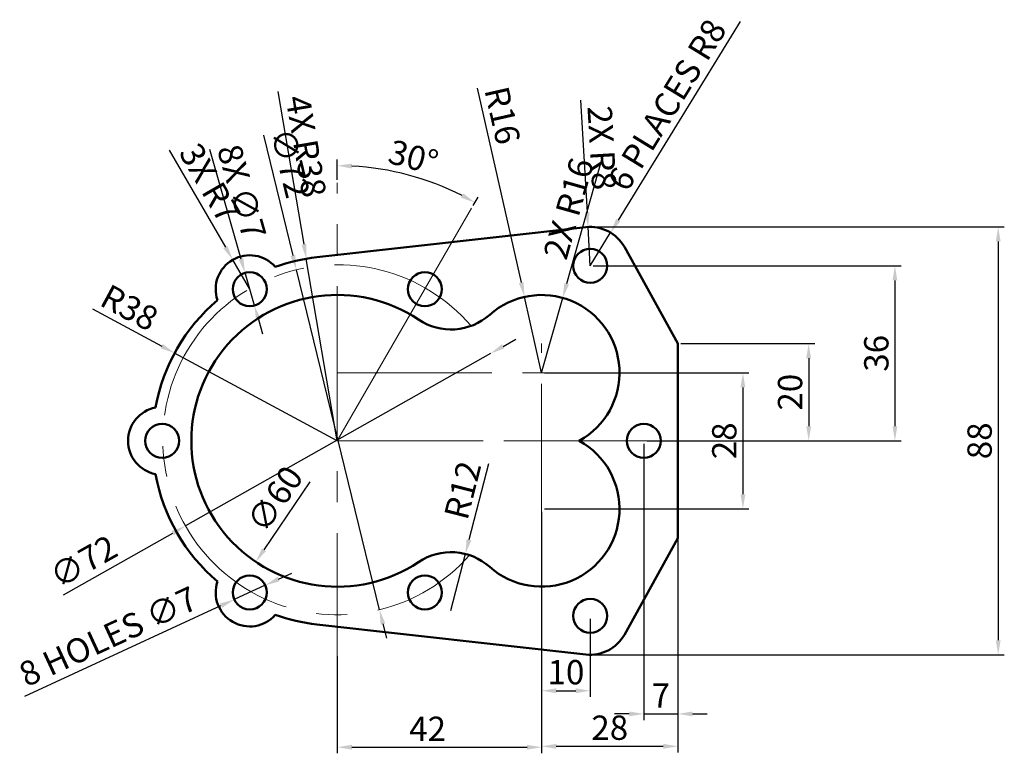
# Model space of a CAD drawing. Units: millimetres. Extents: x 620 to 823, y 325 to 476.
import ezdxf

# ---------------------------------------------------------------- set-up
doc = ezdxf.new("R2010")
doc.units = ezdxf.units.MM
doc.linetypes.add('CENTER', pattern=[50.8, 31.75, -6.35, 6.35, -6.35])
for name, color, linetype, lineweight in [('M-CNTR', 4, 'CENTER', 18), ('M-CONS', 8, 'Continuous', 18), ('M-DIMS', 2, 'Continuous', 25), ('M-OUTL', 7, 'Continuous', 50)]:
    doc.layers.add(name, color=color, linetype=linetype, lineweight=lineweight)
doc.styles.get("Standard").update_dxf_attribs({"font": 'arial.ttf'})
doc.dimstyles.new('ISO-25', dxfattribs={"dimtxt": 5, "dimasz": 3, "dimexe": 1.25, "dimexo": 0.625, "dimtad": 1, "dimdec": 0, "dimtxsty": 'Standard', "dimcen": 2.5, "dimadec": 0, "dimazin": 0, "dimtfac": 1, "dimtdec": 0, "dimtmove": 0, "dimatfit": 3, "dimfxl": 1, "dimarcsym": 0})

# ---------------------------------------------------------------- blocks, each defined once
blk = doc.blocks.new('*D1')
at = {"layer": 'Defpoints', "color": 0, "transparency": 16777216}
for p in [(737.47, 433.5), (737.47, 345.5), (821.32, 345.5)]:
    blk.add_point(p, dxfattribs=at)
at = {"layer": 'M-DIMS', "color": 0, "lineweight": -2, "transparency": 16777216}
for p, q in [((738.09, 433.5), (822.57, 433.5)), ((821.32, 430.5), (821.32, 348.5)), ((738.09, 345.5), (822.57, 345.5))]:
    blk.add_line(p, q, dxfattribs=at)
at = {"layer": 'M-DIMS', "color": 0, "transparency": 16777216}
for points in [[(820.82, 430.5), (821.82, 430.5), (821.32, 433.5)], [(820.82, 348.5), (821.82, 348.5), (821.32, 345.5)]]:
    blk.add_solid(points, dxfattribs=at)
at = {"layer": 'M-DIMS', "color": 0, "transparency": 16777216, "insert": (818.14, 389.5), "char_height": 5, "attachment_point": 5, "rotation": 90}
blk.add_mtext('88', dxfattribs=at)
blk = doc.blocks.new('*D2')
at = {"layer": 'Defpoints', "color": 0, "transparency": 16777216}
for p in [(737.47, 425.5), (748.54, 389.5), (800.09, 389.5)]:
    blk.add_point(p, dxfattribs=at)
at = {"layer": 'M-DIMS', "color": 0, "lineweight": -2, "transparency": 16777216}
for p, q in [((738.09, 425.5), (801.34, 425.5)), ((800.09, 422.5), (800.09, 392.5)), ((749.16, 389.5), (801.34, 389.5))]:
    blk.add_line(p, q, dxfattribs=at)
at = {"layer": 'M-DIMS', "color": 0, "transparency": 16777216}
for points in [[(799.59, 422.5), (800.59, 422.5), (800.09, 425.5)], [(799.59, 392.5), (800.59, 392.5), (800.09, 389.5)]]:
    blk.add_solid(points, dxfattribs=at)
at = {"layer": 'M-DIMS', "color": 0, "transparency": 16777216, "insert": (796.91, 407.5), "char_height": 5, "attachment_point": 5, "rotation": 90}
blk.add_mtext('36', dxfattribs=at)
blk = doc.blocks.new('*D3')
at = {"layer": 'Defpoints', "color": 0, "transparency": 16777216}
for p in [(727.47, 375.5), (685.47, 345.82), (727.47, 326.48)]:
    blk.add_point(p, dxfattribs=at)
at = {"layer": 'M-DIMS', "color": 0, "lineweight": -2, "transparency": 16777216}
for p, q in [((727.47, 374.87), (727.47, 325.23)), ((685.47, 345.2), (685.47, 325.23)), ((688.47, 326.48), (724.47, 326.48))]:
    blk.add_line(p, q, dxfattribs=at)
at = {"layer": 'M-DIMS', "color": 0, "transparency": 16777216}
for points in [[(688.47, 326.98), (688.47, 325.98), (685.47, 326.48)], [(724.47, 326.98), (724.47, 325.98), (727.47, 326.48)]]:
    blk.add_solid(points, dxfattribs=at)
at = {"layer": 'M-DIMS', "color": 0, "transparency": 16777216, "insert": (704.03, 329.62), "char_height": 5, "attachment_point": 5}
blk.add_mtext('42', dxfattribs=at)
blk = doc.blocks.new('*D4')
at = {"layer": 'Defpoints', "color": 0, "transparency": 16777216}
for p in [(755.47, 409.5), (763.47, 389.5), (782.36, 389.5)]:
    blk.add_point(p, dxfattribs=at)
at = {"layer": 'M-DIMS', "color": 0, "lineweight": -2, "transparency": 16777216}
for p, q in [((756.09, 409.5), (783.61, 409.5)), ((782.36, 406.5), (782.36, 392.5)), ((764.09, 389.5), (783.61, 389.5))]:
    blk.add_line(p, q, dxfattribs=at)
at = {"layer": 'M-DIMS', "color": 0, "transparency": 16777216}
for points in [[(781.86, 406.5), (782.86, 406.5), (782.36, 409.5)], [(781.86, 392.5), (782.86, 392.5), (782.36, 389.5)]]:
    blk.add_solid(points, dxfattribs=at)
at = {"layer": 'M-DIMS', "color": 0, "transparency": 16777216, "insert": (779.18, 399.5), "char_height": 5, "attachment_point": 5, "rotation": 90}
blk.add_mtext('20', dxfattribs=at)
blk = doc.blocks.new('*D5')
at = {"layer": 'Defpoints', "color": 0, "transparency": 16777216}
for p in [(727.47, 403.5), (727.47, 375.5), (768.84, 375.5)]:
    blk.add_point(p, dxfattribs=at)
at = {"layer": 'M-DIMS', "color": 0, "lineweight": -2, "transparency": 16777216}
for p, q in [((728.09, 403.5), (770.09, 403.5)), ((768.84, 400.5), (768.84, 378.5)), ((728.09, 375.5), (770.09, 375.5))]:
    blk.add_line(p, q, dxfattribs=at)
at = {"layer": 'M-DIMS', "color": 0, "transparency": 16777216}
for points in [[(768.34, 400.5), (769.34, 400.5), (768.84, 403.5)], [(768.34, 378.5), (769.34, 378.5), (768.84, 375.5)]]:
    blk.add_solid(points, dxfattribs=at)
at = {"layer": 'M-DIMS', "color": 0, "transparency": 16777216, "insert": (765.66, 389.5), "char_height": 5, "attachment_point": 5, "rotation": 90}
blk.add_mtext('28', dxfattribs=at)
blk = doc.blocks.new('*D6')
at = {"layer": 'Defpoints', "color": 0, "transparency": 16777216}
for p in [(748.47, 389.5), (755.47, 383.53), (755.47, 333.33)]:
    blk.add_point(p, dxfattribs=at)
at = {"layer": 'M-DIMS', "color": 0, "lineweight": -2, "transparency": 16777216}
for p, q in [((748.47, 388.87), (748.47, 332.08)), ((755.47, 382.9), (755.47, 332.08)), ((745.47, 333.33), (742.47, 333.33)), ((748.47, 333.33), (755.47, 333.33)), ((758.47, 333.33), (761.47, 333.33))]:
    blk.add_line(p, q, dxfattribs=at)
at = {"layer": 'M-DIMS', "color": 0, "transparency": 16777216}
for points in [[(745.47, 333.83), (745.47, 332.83), (748.47, 333.33)], [(758.47, 333.83), (758.47, 332.83), (755.47, 333.33)]]:
    blk.add_solid(points, dxfattribs=at)
at = {"layer": 'M-DIMS', "color": 0, "transparency": 16777216, "insert": (751.97, 336.46), "char_height": 5, "attachment_point": 5}
blk.add_mtext('7', dxfattribs=at)
blk = doc.blocks.new('*D7')
at = {"layer": 'Defpoints', "color": 0, "transparency": 16777216}
for p in [(737.47, 353.5), (727.47, 344.51), (737.47, 338.1)]:
    blk.add_point(p, dxfattribs=at)
at = {"layer": 'M-DIMS', "color": 0, "lineweight": -2, "transparency": 16777216}
for p, q in [((737.47, 352.87), (737.47, 336.85)), ((727.47, 343.88), (727.47, 336.85)), ((730.47, 338.1), (734.47, 338.1))]:
    blk.add_line(p, q, dxfattribs=at)
at = {"layer": 'M-DIMS', "color": 0, "transparency": 16777216}
for points in [[(730.47, 338.6), (730.47, 337.6), (727.47, 338.1)], [(734.47, 338.6), (734.47, 337.6), (737.47, 338.1)]]:
    blk.add_solid(points, dxfattribs=at)
at = {"layer": 'M-DIMS', "color": 0, "transparency": 16777216, "insert": (732.47, 341.27), "char_height": 5, "attachment_point": 5}
blk.add_mtext('10', dxfattribs=at)
blk = doc.blocks.new('*D8')
at = {"layer": 'Defpoints', "color": 0, "transparency": 16777216}
for p in [(741.65, 432.32), (737.47, 425.5)]:
    blk.add_point(p, dxfattribs=at)
at = {"layer": 'M-DIMS', "color": 0, "lineweight": -2, "transparency": 16777216}
for p, q in [((768.26, 475.75), (743.21, 434.88)), ((737.47, 425.5), (741.65, 432.32))]:
    blk.add_line(p, q, dxfattribs=at)
at = {"layer": 'M-DIMS', "color": 0, "transparency": 16777216}
blk.add_solid([(742.79, 435.14), (743.64, 434.62), (741.65, 432.32)], dxfattribs=at)
at = {"layer": 'M-DIMS', "color": 0, "transparency": 16777216, "insert": (753.78, 458.27), "char_height": 5, "attachment_point": 5, "rotation": 58.5023}
blk.add_mtext('6 PLACES R8', dxfattribs=at)
blk = doc.blocks.new('*D9')
at = {"layer": 'Defpoints', "color": 0, "transparency": 16777216}
for p in [(723.94, 419.1), (727.47, 403.5)]:
    blk.add_point(p, dxfattribs=at)
at = {"layer": 'M-DIMS', "color": 0, "lineweight": -2, "transparency": 16777216}
for p, q in [((714.23, 462.03), (723.28, 422.03)), ((727.47, 403.5), (723.94, 419.1))]:
    blk.add_line(p, q, dxfattribs=at)
at = {"layer": 'M-DIMS', "color": 0, "transparency": 16777216}
blk.add_solid([(723.76, 422.14), (722.79, 421.92), (723.94, 419.1)], dxfattribs=at)
at = {"layer": 'M-DIMS', "color": 0, "transparency": 16777216, "insert": (718.79, 456.3), "char_height": 5, "attachment_point": 5, "rotation": 282.7415}
blk.add_mtext('R16', dxfattribs=at)
blk = doc.blocks.new('*D10')
at = {"layer": 'Defpoints', "color": 0, "transparency": 16777216}
for p in [(711.79, 366.23), (708.83, 354.6)]:
    blk.add_point(p, dxfattribs=at)
at = {"layer": 'M-DIMS', "color": 0, "lineweight": -2, "transparency": 16777216}
for p, q in [((716.52, 384.78), (712.53, 369.13)), ((708.83, 354.6), (711.79, 366.23))]:
    blk.add_line(p, q, dxfattribs=at)
at = {"layer": 'M-DIMS', "color": 0, "transparency": 16777216}
blk.add_solid([(712.05, 369.26), (713.02, 369.01), (711.79, 366.23)], dxfattribs=at)
at = {"layer": 'M-DIMS', "color": 0, "transparency": 16777216, "insert": (711.86, 379.18), "char_height": 5, "attachment_point": 5, "rotation": 75.7174}
blk.add_mtext('R12', dxfattribs=at)
blk = doc.blocks.new('*D11')
at = {"layer": 'Defpoints', "color": 0, "transparency": 16777216}
for p in [(652.03, 407.54), (685.47, 389.5)]:
    blk.add_point(p, dxfattribs=at)
at = {"layer": 'M-DIMS', "color": 0, "lineweight": -2, "transparency": 16777216}
for p, q in [((635.12, 416.67), (649.39, 408.97)), ((685.47, 389.5), (652.03, 407.54))]:
    blk.add_line(p, q, dxfattribs=at)
at = {"layer": 'M-DIMS', "color": 0, "transparency": 16777216}
blk.add_solid([(649.62, 409.41), (649.15, 408.53), (652.03, 407.54)], dxfattribs=at)
at = {"layer": 'M-DIMS', "color": 0, "transparency": 16777216, "insert": (642.44, 416.33), "char_height": 5, "attachment_point": 5, "rotation": 331.6462}
blk.add_mtext('R38', dxfattribs=at)
blk = doc.blocks.new('*D12')
at = {"layer": 'Defpoints', "color": 0, "transparency": 16777216}
for p in [(716.93, 407.44), (654.26, 371.99)]:
    blk.add_point(p, dxfattribs=at)
at = {"layer": 'M-DIMS', "color": 0, "lineweight": -2, "transparency": 16777216}
for p, q in [((719.54, 408.92), (722.15, 410.4)), ((716.93, 407.44), (654.26, 371.99)), ((629.21, 357.82), (651.65, 370.52))]:
    blk.add_line(p, q, dxfattribs=at)
at = {"layer": 'M-DIMS', "color": 0, "transparency": 16777216}
for points in [[(719.29, 409.36), (719.79, 408.49), (716.93, 407.44)], [(651.4, 370.95), (651.9, 370.08), (654.26, 371.99)]]:
    blk.add_solid(points, dxfattribs=at)
at = {"layer": 'M-DIMS', "color": 0, "transparency": 16777216, "insert": (633.59, 364.11), "char_height": 5, "attachment_point": 5, "rotation": 29.4967}
blk.add_mtext('∅72', dxfattribs=at)
blk = doc.blocks.new('*D13')
at = {"layer": 'Defpoints', "color": 0, "transparency": 16777216}
for p in [(702.22, 414.39), (668.72, 364.61)]:
    blk.add_point(p, dxfattribs=at)
at = {"layer": 'M-DIMS', "color": 0, "lineweight": -2, "transparency": 16777216}
blk.add_line((679.79, 381.06), (670.39, 367.1), dxfattribs=at)
at = {"layer": 'M-DIMS', "color": 0, "transparency": 16777216}
blk.add_solid([(669.98, 367.38), (670.81, 366.82), (668.72, 364.61)], dxfattribs=at)
at = {"layer": 'M-DIMS', "color": 0, "transparency": 16777216, "insert": (673.18, 377.18), "char_height": 5, "attachment_point": 5, "rotation": 56.0608}
blk.add_mtext('∅60', dxfattribs=at)
blk = doc.blocks.new('*D14')
at = {"layer": 'Defpoints', "color": 0, "transparency": 16777216}
for p in [(670.65, 359.79), (664.29, 356.86)]:
    blk.add_point(p, dxfattribs=at)
at = {"layer": 'M-DIMS', "color": 0, "lineweight": -2, "transparency": 16777216}
for p, q in [((673.37, 361.04), (676.1, 362.3)), ((670.65, 359.79), (664.29, 356.86)), ((621.23, 337.01), (661.56, 355.6))]:
    blk.add_line(p, q, dxfattribs=at)
at = {"layer": 'M-DIMS', "color": 0, "transparency": 16777216}
for points in [[(673.16, 361.5), (673.58, 360.59), (670.65, 359.79)], [(661.35, 356.05), (661.77, 355.15), (664.29, 356.86)]]:
    blk.add_solid(points, dxfattribs=at)
at = {"layer": 'M-DIMS', "color": 0, "transparency": 16777216, "insert": (638.65, 348.69), "char_height": 5, "attachment_point": 5, "rotation": 24.7445}
blk.add_mtext('8 HOLES ∅7', dxfattribs=at)
blk = doc.blocks.new('*D15')
at = {"layer": 'Defpoints', "color": 0, "transparency": 16777216}
for p in [(685.47, 442.56), (704.82, 442.68), (713.08, 437.33), (685.47, 389.5), (685.47, 338.78)]:
    blk.add_point(p, dxfattribs=at)
at = {"layer": 'M-DIMS', "color": 0, "lineweight": -2, "transparency": 16777216}
for p, q in [((685.47, 443.18), (685.47, 447.34)), ((713.39, 437.87), (714.39, 439.59))]:
    blk.add_line(p, q, dxfattribs=at)
blk.add_arc((685.47, 389.5), 56.59, 63.0377, 86.9623, dxfattribs=at)
at = {"layer": 'M-DIMS', "color": 0, "transparency": 16777216}
for points in [[(688.45, 445.51), (688.48, 446.51), (685.47, 446.09)], [(711.36, 440.38), (710.89, 439.5), (713.76, 438.51)]]:
    blk.add_solid(points, dxfattribs=at)
at = {"layer": 'M-DIMS', "color": 0, "transparency": 16777216, "insert": (700.94, 447.23), "char_height": 5, "attachment_point": 5, "rotation": 345}
blk.add_mtext('30°', dxfattribs=at)
blk = doc.blocks.new('*D16')
at = {"layer": 'Defpoints', "color": 0, "transparency": 16777216}
for p in [(727.47, 343.1), (755.47, 343.1), (755.47, 326.67)]:
    blk.add_point(p, dxfattribs=at)
at = {"layer": 'M-DIMS', "color": 0, "lineweight": -2, "transparency": 16777216}
for p, q in [((727.47, 342.48), (727.47, 325.42)), ((755.47, 342.48), (755.47, 325.42)), ((730.47, 326.67), (752.47, 326.67))]:
    blk.add_line(p, q, dxfattribs=at)
at = {"layer": 'M-DIMS', "color": 0, "transparency": 16777216}
for points in [[(730.47, 327.17), (730.47, 326.17), (727.47, 326.67)], [(752.47, 327.17), (752.47, 326.17), (755.47, 326.67)]]:
    blk.add_solid(points, dxfattribs=at)
at = {"layer": 'M-DIMS', "color": 0, "transparency": 16777216, "insert": (741.47, 329.85), "char_height": 5, "attachment_point": 5}
blk.add_mtext('28', dxfattribs=at)
blk = doc.blocks.new('BOLT-HOLE-D7')
blk.add_circle((3.5, 3.5), 3.5)
blk = doc.blocks.new('*D18')
at = {"layer": 'Defpoints', "color": 0, "transparency": 16777216}
for p in [(666.5, 424.04), (668.43, 417.31)]:
    blk.add_point(p, dxfattribs=at)
at = {"layer": 'M-DIMS', "color": 0, "lineweight": -2, "transparency": 16777216}
for p, q in [((659.19, 449.46), (665.67, 426.92)), ((668.43, 417.31), (666.5, 424.04)), ((669.26, 414.43), (670.09, 411.54))]:
    blk.add_line(p, q, dxfattribs=at)
at = {"layer": 'M-DIMS', "color": 0, "transparency": 16777216}
for points in [[(666.15, 427.06), (665.19, 426.78), (666.5, 424.04)], [(669.74, 414.57), (668.78, 414.29), (668.43, 417.31)]]:
    blk.add_solid(points, dxfattribs=at)
at = {"layer": 'M-DIMS', "color": 0, "transparency": 16777216, "insert": (665.21, 440.55), "char_height": 5, "attachment_point": 5, "rotation": 286.0373}
blk.add_mtext('8X ∅7', dxfattribs=at)
blk = doc.blocks.new('*D19')
at = {"layer": 'Defpoints', "color": 0, "transparency": 16777216}
for p in [(663.97, 426.74), (667.47, 420.67)]:
    blk.add_point(p, dxfattribs=at)
at = {"layer": 'M-DIMS', "color": 0, "lineweight": -2, "transparency": 16777216}
for p, q in [((650.94, 449.3), (662.47, 429.33)), ((667.47, 420.67), (663.97, 426.74))]:
    blk.add_line(p, q, dxfattribs=at)
at = {"layer": 'M-DIMS', "color": 0, "transparency": 16777216}
blk.add_solid([(662.9, 429.58), (662.03, 429.08), (663.97, 426.74)], dxfattribs=at)
at = {"layer": 'M-DIMS', "color": 0, "transparency": 16777216, "insert": (658.71, 442.21), "char_height": 5, "attachment_point": 5, "rotation": 300.0017}
blk.add_mtext('3X R7', dxfattribs=at)
blk = doc.blocks.new('*D20')
at = {"layer": 'Defpoints', "color": 0, "transparency": 16777216}
for p in [(737, 433.48), (737.47, 425.5)]:
    blk.add_point(p, dxfattribs=at)
at = {"layer": 'M-DIMS', "color": 0, "lineweight": -2, "transparency": 16777216}
for p, q in [((735.47, 459.59), (736.82, 436.48)), ((737.47, 425.5), (737, 433.48))]:
    blk.add_line(p, q, dxfattribs=at)
at = {"layer": 'M-DIMS', "color": 0, "transparency": 16777216}
blk.add_solid([(737.32, 436.51), (736.33, 436.45), (737, 433.48)], dxfattribs=at)
at = {"layer": 'M-DIMS', "color": 0, "transparency": 16777216, "insert": (739.23, 449.72), "char_height": 5, "attachment_point": 5, "rotation": 273.351}
blk.add_mtext('2X R8', dxfattribs=at)
blk = doc.blocks.new('*D21')
at = {"layer": 'Defpoints', "color": 0, "transparency": 16777216}
for p in [(679.1, 426.96), (685.47, 389.5)]:
    blk.add_point(p, dxfattribs=at)
at = {"layer": 'M-DIMS', "color": 0, "lineweight": -2, "transparency": 16777216}
for p, q in [((673.25, 461.34), (678.6, 429.92)), ((685.47, 389.5), (679.1, 426.96))]:
    blk.add_line(p, q, dxfattribs=at)
at = {"layer": 'M-DIMS', "color": 0, "transparency": 16777216}
blk.add_solid([(679.09, 430), (678.1, 429.83), (679.1, 426.96)], dxfattribs=at)
at = {"layer": 'M-DIMS', "color": 0, "transparency": 16777216, "insert": (678.41, 449.97), "char_height": 5, "attachment_point": 5, "rotation": 279.6488}
blk.add_mtext('4X R38', dxfattribs=at)
blk = doc.blocks.new('*D22')
at = {"layer": 'Defpoints', "color": 0, "transparency": 16777216}
for p in [(677.05, 424.69), (694.14, 354.75)]:
    blk.add_point(p, dxfattribs=at)
at = {"layer": 'M-DIMS', "color": 0, "lineweight": -2, "transparency": 16777216}
for p, q in [((670.29, 452.38), (676.34, 427.6)), ((694.14, 354.75), (677.05, 424.69)), ((694.85, 351.83), (695.56, 348.92))]:
    blk.add_line(p, q, dxfattribs=at)
at = {"layer": 'M-DIMS', "color": 0, "transparency": 16777216}
for points in [[(676.82, 427.72), (675.85, 427.49), (677.05, 424.69)], [(695.34, 351.95), (694.37, 351.71), (694.14, 354.75)]]:
    blk.add_solid(points, dxfattribs=at)
at = {"layer": 'M-DIMS', "color": 0, "transparency": 16777216, "insert": (675.15, 446.46), "char_height": 5, "attachment_point": 5, "rotation": 283.7292}
blk.add_mtext('∅72', dxfattribs=at)
blk = doc.blocks.new('*D23')
at = {"layer": 'Defpoints', "color": 0, "transparency": 16777216}
for p in [(731.8, 418.9), (727.47, 403.5)]:
    blk.add_point(p, dxfattribs=at)
at = {"layer": 'M-DIMS', "color": 0, "lineweight": -2, "transparency": 16777216}
for p, q in [((739.93, 447.8), (732.61, 421.79)), ((727.47, 403.5), (731.8, 418.9))]:
    blk.add_line(p, q, dxfattribs=at)
at = {"layer": 'M-DIMS', "color": 0, "transparency": 16777216}
blk.add_solid([(732.13, 421.92), (733.09, 421.65), (731.8, 418.9)], dxfattribs=at)
at = {"layer": 'M-DIMS', "color": 0, "transparency": 16777216, "insert": (733.62, 437.1), "char_height": 5, "attachment_point": 5, "rotation": 74.289}
blk.add_mtext('2X R16', dxfattribs=at)

msp = doc.modelspace()

# ---------------------------------------------------------------- linework, layer by layer
at = {"layer": 'M-CNTR'}
for p, q in [((685.47, 338.78), (685.47, 442.56)), ((727.47, 369.5), (727.47, 409.5)), ((685.47, 403.5), (755.47, 403.5))]:
    msp.add_line(p, q, dxfattribs=at)
msp.add_arc((685.6, 389.72), 36, 40.5534, 318.7313, dxfattribs=at)
at = {"layer": 'M-CONS'}
for p, q in [((685.47, 389.5), (713.08, 437.33)), ((685.47, 389.5), (715.47, 389.5)), ((719.72, 389.5), (755.47, 389.5))]:
    msp.add_line(p, q, dxfattribs=at)
at = {"layer": 'M-OUTL'}
for p, q in [((736.58, 433.45), (681.25, 427.26)), ((744.47, 429.37), (755.47, 409.5)), ((755.47, 369.5), (755.47, 409.5)), ((744.47, 349.62), (755.47, 369.5)), ((736.58, 345.55), (681.25, 351.73))]:
    msp.add_line(p, q, dxfattribs=at)
for centre, radius, start, end in [((737.47, 425.5), 8, 28.9652, 96.3787), ((667.47, 420.67), 7, 41.3282, 198.6718), ((685.47, 389.5), 38, 96.3787, 109.594), ((685.47, 389.5), 30, 56.1962, 303.8038), ((727.47, 403.5), 16, 298.955, 131.7187), ((685.47, 389.5), 38, 130.406, 169.594), ((708.83, 424.4), 12, 236.1962, 311.7187), ((649.47, 389.5), 7, 101.3282, 258.6718), ((727.47, 375.5), 16, 228.2813, 61.045), ((685.47, 389.5), 38, 190.406, 229.594), ((708.83, 354.6), 12, 48.2813, 123.8038), ((667.47, 358.32), 7, 161.3282, 318.6718), ((685.47, 389.5), 38, 250.406, 263.6213), ((737.47, 353.5), 8, 263.6213, 331.0348)]:
    msp.add_arc(centre, radius, start, end, dxfattribs=at)

# ---------------------------------------------------------------- block references
for p in [(733.97, 422), (663.97, 417.18), (699.97, 417.18), (645.97, 386), (744.97, 386), (663.97, 354.82), (699.97, 354.82), (733.97, 350)]:
    msp.add_blockref('BOLT-HOLE-D7', p, dxfattribs=at)

# ---------------------------------------------------------------- dimensions: what is measured, and where the dimension line sits
at = {"layer": 'M-DIMS'}
for center, mpoint, text, override, picture, middle in [((737.47, 425.5), (741.65, 432.32), '6 PLACES <>', {"dimclrd": 0, "dimclre": 0, "dimclrt": 0}, '*D8', (753.78, 458.27)), ((737.47, 425.5), (737, 433.48), '2X <>', {"dimdec": 0, "dimlfac": 1, "dimrnd": 0, "dimzin": 0, "dimdsep": 46, "dimlunit": 2}, '*D20', (739.23, 449.72)), ((667.47, 420.67), (663.97, 426.74), '3X <>', {"dimdec": 0, "dimlfac": 1, "dimrnd": 0, "dimzin": 0, "dimdsep": 46, "dimlunit": 2}, '*D19', (658.71, 442.21)), ((727.47, 403.5), (731.8, 418.9), '2X <>', {"dimdec": 0, "dimlfac": 1, "dimrnd": 0, "dimzin": 0, "dimdsep": 46, "dimlunit": 2}, '*D23', (733.62, 437.1))]:
    dim = msp.add_radius_dim(center=center, mpoint=mpoint, text=text, dimstyle='ISO-25', override=override, dxfattribs=at)
    dim.commit()
    dim.dimension.update_dxf_attribs({"geometry": picture, "text_midpoint": middle})
dim = msp.add_radius_dim(center=(727.47, 403.5), mpoint=(723.94, 419.1), dimstyle='ISO-25', override={"dimclrd": 0, "dimclre": 0, "dimclrt": 0}, dxfattribs=at)
dim.commit()
dim.dimension.update_dxf_attribs({"geometry": '*D9', "text_midpoint": (715.69, 455.6), "dimtype": 164})
dim = msp.add_radius_dim(center=(685.47, 389.5), mpoint=(679.1, 426.96), text='4X <>', dimstyle='ISO-25', override={"dimdec": 0, "dimlfac": 1, "dimrnd": 0, "dimzin": 0, "dimdsep": 46, "dimlunit": 2}, dxfattribs=at)
dim.commit()
dim.dimension.update_dxf_attribs({"geometry": '*D21', "text_midpoint": (675.28, 449.44), "dimtype": 164})
for p1, p2, override, picture, middle in [((694.14, 354.75), (677.05, 424.69), {"dimdec": 0, "dimlfac": 1, "dimrnd": 0, "dimzin": 0, "dimdsep": 46, "dimlunit": 2}, '*D22', (671.92, 445.67)), ((702.22, 414.39), (668.72, 364.61), {"dimclrd": 0, "dimclre": 0, "dimclrt": 0}, '*D13', (675.93, 375.33)), ((716.93, 407.44), (654.26, 371.99), {"dimclrd": 0, "dimclre": 0, "dimclrt": 0}, '*D12', (635.22, 361.22))]:
    dim = msp.add_diameter_dim_2p(p1=p1, p2=p2, dimstyle='ISO-25', override=override, dxfattribs=at)
    dim.commit()
    dim.dimension.update_dxf_attribs({"geometry": picture, "text_midpoint": middle, "dimtype": 163})
dim = msp.add_angular_dim_2l(base=(704.82, 442.68), line1=((685.47, 338.78), (685.47, 442.56)), line2=((685.47, 389.5), (713.08, 437.33)), dimstyle='ISO-25', override={"dimclrd": 0, "dimclre": 0, "dimclrt": 0}, dxfattribs=at)
dim.commit()
dim.dimension.update_dxf_attribs({"geometry": '*D15', "text_midpoint": (700.94, 447.23)})
for p1, p2, text, override, picture, middle in [((668.43, 417.31), (666.5, 424.04), '8X <>', {"dimdec": 0, "dimlfac": 1, "dimrnd": 0, "dimzin": 0, "dimdsep": 46, "dimlunit": 2}, '*D18', (662.02, 439.63)), ((670.65, 359.79), (664.29, 356.86), '8 HOLES <>', {"dimclrd": 0, "dimclre": 0, "dimclrt": 0}, '*D14', (638.65, 348.69))]:
    dim = msp.add_diameter_dim_2p(p1=p1, p2=p2, text=text, dimstyle='ISO-25', override=override, dxfattribs=at)
    dim.commit()
    dim.dimension.update_dxf_attribs({"geometry": picture, "text_midpoint": middle})
for base, p1, p2, picture, middle in [((821.32, 345.5), (737.47, 433.5), (737.47, 345.5), '*D1', (818.14, 389.5)), ((800.09, 389.5), (737.47, 425.5), (748.54, 389.5), '*D2', (796.91, 407.5)), ((782.36, 389.5), (755.47, 409.5), (763.47, 389.5), '*D4', (779.18, 399.5)), ((768.84, 375.5), (727.47, 403.5), (727.47, 375.5), '*D5', (765.66, 389.5))]:
    dim = msp.add_linear_dim(base=base, p1=p1, p2=p2, angle=90, dimstyle='ISO-25', override={"dimclrd": 0, "dimclre": 0, "dimclrt": 0}, dxfattribs=at)
    dim.commit()
    dim.dimension.update_dxf_attribs({"geometry": picture, "text_midpoint": middle})
for center, mpoint, picture, middle in [((685.47, 389.5), (652.03, 407.54), '*D11', (642.44, 416.33)), ((708.83, 354.6), (711.79, 366.23), '*D10', (711.86, 379.18))]:
    dim = msp.add_radius_dim(center=center, mpoint=mpoint, dimstyle='ISO-25', override={"dimclrd": 0, "dimclre": 0, "dimclrt": 0}, dxfattribs=at)
    dim.commit()
    dim.dimension.update_dxf_attribs({"geometry": picture, "text_midpoint": middle})
for base, p1, p2, picture, middle in [((755.47, 333.33), (748.47, 389.5), (755.47, 383.53), '*D6', (751.97, 336.46)), ((737.47, 338.1), (727.47, 344.51), (737.47, 353.5), '*D7', (732.47, 341.27)), ((755.47, 326.67), (727.47, 343.1), (755.47, 343.1), '*D16', (741.47, 329.85))]:
    dim = msp.add_linear_dim(base=base, p1=p1, p2=p2, dimstyle='ISO-25', override={"dimclrd": 0, "dimclre": 0, "dimclrt": 0}, dxfattribs=at)
    dim.commit()
    dim.dimension.update_dxf_attribs({"geometry": picture, "text_midpoint": middle})
dim = msp.add_linear_dim(base=(727.47, 326.48), p1=(685.47, 345.82), p2=(727.47, 375.5), dimstyle='ISO-25', override={"dimclrd": 0, "dimclre": 0, "dimclrt": 0}, dxfattribs=at)
dim.commit()
dim.dimension.update_dxf_attribs({"geometry": '*D3', "text_midpoint": (704.03, 326.48), "dimtype": 160})

doc.saveas('drawing.dxf')
